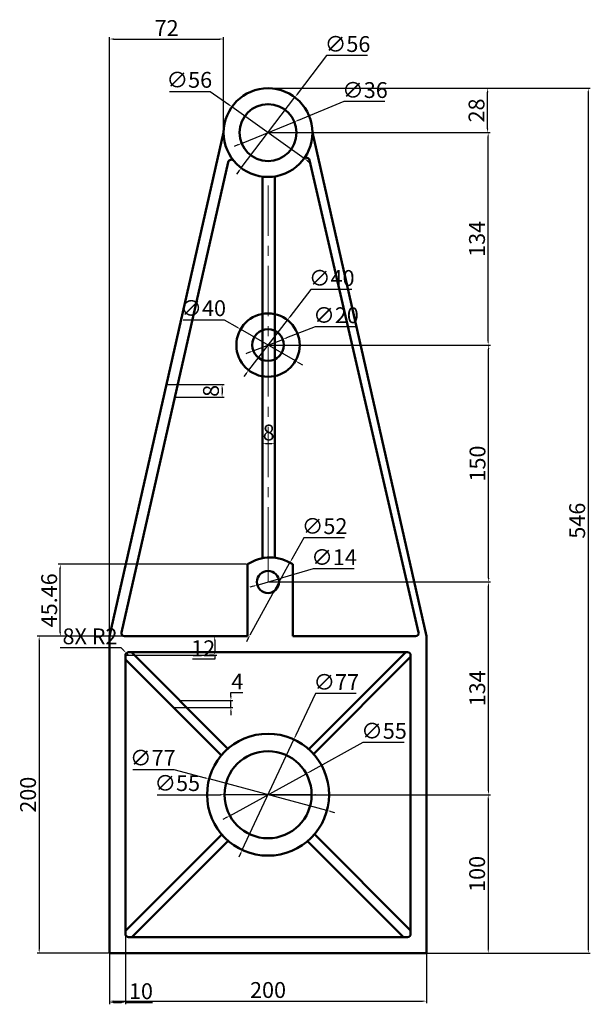
# Model space of a CAD drawing. Units: millimetres. Extents: x 2478 to 2838, y 972 to 1594.
import ezdxf

# ---------------------------------------------------------------- set-up
doc = ezdxf.new("R2010")
doc.units = ezdxf.units.MM
doc.linetypes.add('CENTER', pattern=[50.8, 31.75, -6.35, 6.35, -6.35])
for name, color, linetype, lineweight in [('M-CNTR', 4, 'CENTER', 18), ('M-DIMS', 2, 'Continuous', 25), ('M-OUTL', 7, 'Continuous', 50)]:
    doc.layers.add(name, color=color, linetype=linetype, lineweight=lineweight)
doc.styles.get("Standard").update_dxf_attribs({"font": 'arial.ttf'})
doc.dimstyles.new('ISO-25', dxfattribs={"dimtxt": 10, "dimasz": 2.5, "dimexe": 1.25, "dimexo": 0.625, "dimtad": 1, "dimtoh": 1, "dimdec": 0, "dimtxsty": 'Standard', "dimcen": 2.5, "dimadec": 0, "dimazin": 0, "dimtfac": 1, "dimtdec": 0, "dimtmove": 0, "dimatfit": 3, "dimfxl": 1, "dimarcsym": 0})

# ---------------------------------------------------------------- blocks, each defined once
blk = doc.blocks.new('*D1')
at = {"layer": 'Defpoints', "color": 0, "transparency": 16777216}
for p in [(2651.8, 1544.92), (2617.92, 1500.33)]:
    blk.add_point(p, dxfattribs=at)
at = {"layer": 'M-DIMS', "color": 0, "lineweight": -2, "transparency": 16777216}
for p, q in [((2671.81, 1571.25), (2653.31, 1546.91)), ((2697.63, 1571.25), (2671.81, 1571.25)), ((2617.92, 1500.33), (2651.8, 1544.92)), ((2616.4, 1498.34), (2614.89, 1496.35))]:
    blk.add_line(p, q, dxfattribs=at)
at = {"layer": 'M-DIMS', "color": 0, "transparency": 16777216}
for points in [[(2652.98, 1547.16), (2653.65, 1546.66), (2651.8, 1544.92)], [(2616.07, 1498.59), (2616.74, 1498.09), (2617.92, 1500.33)]]:
    blk.add_solid(points, dxfattribs=at)
at = {"layer": 'M-DIMS', "color": 0, "transparency": 16777216, "insert": (2685.04, 1577.26), "char_height": 10, "attachment_point": 5}
blk.add_mtext('∅56', dxfattribs=at)
blk = doc.blocks.new('*D2')
at = {"layer": 'Defpoints', "color": 0, "transparency": 16777216}
for p in [(2651.52, 1529.43), (2618.2, 1515.82)]:
    blk.add_point(p, dxfattribs=at)
at = {"layer": 'M-DIMS', "color": 0, "lineweight": -2, "transparency": 16777216}
for p, q in [((2682.79, 1542.2), (2653.84, 1530.38)), ((2708.61, 1542.2), (2682.79, 1542.2)), ((2618.2, 1515.82), (2651.52, 1529.43)), ((2615.88, 1514.87), (2613.57, 1513.93))]:
    blk.add_line(p, q, dxfattribs=at)
at = {"layer": 'M-DIMS', "color": 0, "transparency": 16777216}
for points in [[(2653.68, 1530.76), (2653.99, 1529.99), (2651.52, 1529.43)], [(2615.72, 1515.26), (2616.04, 1514.49), (2618.2, 1515.82)]]:
    blk.add_solid(points, dxfattribs=at)
at = {"layer": 'M-DIMS', "color": 0, "transparency": 16777216, "insert": (2696.01, 1548.21), "char_height": 10, "attachment_point": 5}
blk.add_mtext('∅36', dxfattribs=at)
blk = doc.blocks.new('*D3')
at = {"layer": 'Defpoints', "color": 0, "transparency": 16777216}
for p in [(2647.06, 1404.32), (2622.66, 1372.63)]:
    blk.add_point(p, dxfattribs=at)
at = {"layer": 'M-DIMS', "color": 0, "lineweight": -2, "transparency": 16777216}
for p, q in [((2661.86, 1423.53), (2648.59, 1406.3)), ((2687.65, 1423.53), (2661.86, 1423.53)), ((2622.66, 1372.63), (2647.06, 1404.32)), ((2621.13, 1370.65), (2619.61, 1368.67))]:
    blk.add_line(p, q, dxfattribs=at)
at = {"layer": 'M-DIMS', "color": 0, "transparency": 16777216}
for points in [[(2648.26, 1406.56), (2648.92, 1406.05), (2647.06, 1404.32)], [(2620.8, 1370.9), (2621.46, 1370.39), (2622.66, 1372.63)]]:
    blk.add_solid(points, dxfattribs=at)
at = {"layer": 'M-DIMS', "color": 0, "transparency": 16777216, "insert": (2675.07, 1429.54), "char_height": 10, "attachment_point": 5}
blk.add_mtext('∅40', dxfattribs=at)
blk = doc.blocks.new('*D4')
at = {"layer": 'Defpoints', "color": 0, "transparency": 16777216}
for p in [(2644.18, 1392.1), (2625.54, 1384.85)]:
    blk.add_point(p, dxfattribs=at)
at = {"layer": 'M-DIMS', "color": 0, "lineweight": -2, "transparency": 16777216}
for p, q in [((2664.54, 1400.03), (2646.51, 1393.01)), ((2690.33, 1400.03), (2664.54, 1400.03)), ((2625.54, 1384.85), (2644.18, 1392.1)), ((2623.21, 1383.94), (2620.88, 1383.03))]:
    blk.add_line(p, q, dxfattribs=at)
at = {"layer": 'M-DIMS', "color": 0, "transparency": 16777216}
for points in [[(2646.36, 1393.4), (2646.66, 1392.62), (2644.18, 1392.1)], [(2623.06, 1384.33), (2623.36, 1383.55), (2625.54, 1384.85)]]:
    blk.add_solid(points, dxfattribs=at)
at = {"layer": 'M-DIMS', "color": 0, "transparency": 16777216, "insert": (2677.75, 1406.04), "char_height": 10, "attachment_point": 5}
blk.add_mtext('∅20', dxfattribs=at)
blk = doc.blocks.new('*D5')
at = {"layer": 'Defpoints', "color": 0, "transparency": 16777216}
for p in [(2648.7, 1251.13), (2623.6, 1205.59)]:
    blk.add_point(p, dxfattribs=at)
at = {"layer": 'M-DIMS', "color": 0, "lineweight": -2, "transparency": 16777216}
for p, q in [((2657.37, 1266.87), (2649.9, 1253.32)), ((2683.1, 1266.87), (2657.37, 1266.87)), ((2623.6, 1205.59), (2648.7, 1251.13)), ((2622.39, 1203.4), (2621.18, 1201.21))]:
    blk.add_line(p, q, dxfattribs=at)
at = {"layer": 'M-DIMS', "color": 0, "transparency": 16777216}
for points in [[(2649.54, 1253.52), (2650.27, 1253.12), (2648.7, 1251.13)], [(2622.03, 1203.6), (2622.76, 1203.2), (2623.6, 1205.59)]]:
    blk.add_solid(points, dxfattribs=at)
at = {"layer": 'M-DIMS', "color": 0, "transparency": 16777216, "insert": (2670.55, 1272.88), "char_height": 10, "attachment_point": 5}
blk.add_mtext('∅52', dxfattribs=at)
blk = doc.blocks.new('*D6')
at = {"layer": 'Defpoints', "color": 0, "transparency": 16777216}
for p in [(2641.62, 1240.9), (2628.1, 1236.95)]:
    blk.add_point(p, dxfattribs=at)
at = {"layer": 'M-DIMS', "color": 0, "lineweight": -2, "transparency": 16777216}
for p, q in [((2663.33, 1247.23), (2644.02, 1241.6)), ((2689.12, 1247.23), (2663.33, 1247.23)), ((2628.1, 1236.95), (2641.62, 1240.9)), ((2625.7, 1236.25), (2623.3, 1235.55))]:
    blk.add_line(p, q, dxfattribs=at)
at = {"layer": 'M-DIMS', "color": 0, "transparency": 16777216}
for points in [[(2643.9, 1242), (2644.13, 1241.2), (2641.62, 1240.9)], [(2625.59, 1236.65), (2625.82, 1235.85), (2628.1, 1236.95)]]:
    blk.add_solid(points, dxfattribs=at)
at = {"layer": 'M-DIMS', "color": 0, "transparency": 16777216, "insert": (2676.53, 1253.24), "char_height": 10, "attachment_point": 5}
blk.add_mtext('∅14', dxfattribs=at)
blk = doc.blocks.new('*D7')
at = {"layer": 'Defpoints', "color": 0, "transparency": 16777216}
for p in [(2651.18, 1139.5), (2618.54, 1069.75)]:
    blk.add_point(p, dxfattribs=at)
at = {"layer": 'M-DIMS', "color": 0, "lineweight": -2, "transparency": 16777216}
for p, q in [((2664.71, 1168.41), (2652.24, 1141.76)), ((2690.53, 1168.41), (2664.71, 1168.41)), ((2618.54, 1069.75), (2651.18, 1139.5)), ((2617.48, 1067.49), (2616.42, 1065.22))]:
    blk.add_line(p, q, dxfattribs=at)
at = {"layer": 'M-DIMS', "color": 0, "transparency": 16777216}
for points in [[(2651.86, 1141.94), (2652.61, 1141.58), (2651.18, 1139.5)], [(2617.11, 1067.67), (2617.86, 1067.31), (2618.54, 1069.75)]]:
    blk.add_solid(points, dxfattribs=at)
at = {"layer": 'M-DIMS', "color": 0, "transparency": 16777216, "insert": (2677.93, 1174.42), "char_height": 10, "attachment_point": 5}
blk.add_mtext('∅77', dxfattribs=at)
blk = doc.blocks.new('*D8')
at = {"layer": 'Defpoints', "color": 0, "transparency": 16777216}
for p in [(2658.95, 1117.88), (2610.77, 1091.37)]:
    blk.add_point(p, dxfattribs=at)
at = {"layer": 'M-DIMS', "color": 0, "lineweight": -2, "transparency": 16777216}
for p, q in [((2694.78, 1137.6), (2661.14, 1119.09)), ((2720.68, 1137.6), (2694.78, 1137.6)), ((2610.77, 1091.37), (2658.95, 1117.88)), ((2608.58, 1090.16), (2606.39, 1088.96))]:
    blk.add_line(p, q, dxfattribs=at)
at = {"layer": 'M-DIMS', "color": 0, "transparency": 16777216}
for points in [[(2660.94, 1119.45), (2661.34, 1118.72), (2658.95, 1117.88)], [(2608.38, 1090.53), (2608.78, 1089.8), (2610.77, 1091.37)]]:
    blk.add_solid(points, dxfattribs=at)
at = {"layer": 'M-DIMS', "color": 0, "transparency": 16777216, "insert": (2708.04, 1143.61), "char_height": 10, "attachment_point": 5}
blk.add_mtext('∅55', dxfattribs=at)
blk = doc.blocks.new('*D9')
at = {"layer": 'Defpoints', "color": 0, "transparency": 16777216}
for p in [(2534.86, 1004.62), (2734.86, 1004.62), (2734.86, 974.28)]:
    blk.add_point(p, dxfattribs=at)
at = {"layer": 'M-DIMS', "color": 0, "lineweight": -2, "transparency": 16777216}
for p, q in [((2534.86, 1004), (2534.86, 973.03)), ((2734.86, 1004), (2734.86, 973.03)), ((2537.36, 974.28), (2732.36, 974.28))]:
    blk.add_line(p, q, dxfattribs=at)
at = {"layer": 'M-DIMS', "color": 0, "transparency": 16777216}
for points in [[(2537.36, 974.7), (2537.36, 973.86), (2534.86, 974.28)], [(2732.36, 974.7), (2732.36, 973.86), (2734.86, 974.28)]]:
    blk.add_solid(points, dxfattribs=at)
at = {"layer": 'M-DIMS', "color": 0, "transparency": 16777216, "insert": (2634.86, 980.01), "char_height": 10, "attachment_point": 5}
blk.add_mtext('200', dxfattribs=at)
blk = doc.blocks.new('*D10')
at = {"layer": 'Defpoints', "color": 0, "transparency": 16777216}
for p in [(2534.86, 1204.62), (2490.45, 1004.62), (2534.86, 1004.62)]:
    blk.add_point(p, dxfattribs=at)
at = {"layer": 'M-DIMS', "color": 0, "lineweight": -2, "transparency": 16777216}
for p, q in [((2534.23, 1204.62), (2489.2, 1204.62)), ((2490.45, 1202.12), (2490.45, 1007.12)), ((2534.23, 1004.62), (2489.2, 1004.62))]:
    blk.add_line(p, q, dxfattribs=at)
at = {"layer": 'M-DIMS', "color": 0, "transparency": 16777216}
for points in [[(2490.04, 1202.12), (2490.87, 1202.12), (2490.45, 1204.62)], [(2490.04, 1007.12), (2490.87, 1007.12), (2490.45, 1004.62)]]:
    blk.add_solid(points, dxfattribs=at)
at = {"layer": 'M-DIMS', "color": 0, "transparency": 16777216, "insert": (2484.72, 1104.62), "char_height": 10, "attachment_point": 5, "rotation": 90}
blk.add_mtext('200', dxfattribs=at)
blk = doc.blocks.new('*D11')
at = {"layer": 'Defpoints', "color": 0, "transparency": 16777216}
for p in [(2634.86, 1104.62), (2634.86, 1004.62), (2773.82, 1004.62)]:
    blk.add_point(p, dxfattribs=at)
at = {"layer": 'M-DIMS', "color": 0, "lineweight": -2, "transparency": 16777216}
for p, q in [((2635.48, 1104.62), (2775.07, 1104.62)), ((2773.82, 1102.12), (2773.82, 1007.12)), ((2635.48, 1004.62), (2775.07, 1004.62))]:
    blk.add_line(p, q, dxfattribs=at)
at = {"layer": 'M-DIMS', "color": 0, "transparency": 16777216}
for points in [[(2773.4, 1102.12), (2774.23, 1102.12), (2773.82, 1104.62)], [(2773.4, 1007.12), (2774.23, 1007.12), (2773.82, 1004.62)]]:
    blk.add_solid(points, dxfattribs=at)
at = {"layer": 'M-DIMS', "color": 0, "transparency": 16777216, "insert": (2768.09, 1054.62), "char_height": 10, "attachment_point": 5, "rotation": 90}
blk.add_mtext('100', dxfattribs=at)
blk = doc.blocks.new('*D12')
at = {"layer": 'Defpoints', "color": 0, "transparency": 16777216}
for p in [(2634.86, 1238.92), (2773.94, 1238.92), (2634.86, 1104.62)]:
    blk.add_point(p, dxfattribs=at)
at = {"layer": 'M-DIMS', "color": 0, "lineweight": -2, "transparency": 16777216}
for p, q in [((2635.48, 1238.92), (2775.19, 1238.92)), ((2773.94, 1107.12), (2773.94, 1236.42)), ((2635.48, 1104.62), (2775.19, 1104.62))]:
    blk.add_line(p, q, dxfattribs=at)
at = {"layer": 'M-DIMS', "color": 0, "transparency": 16777216}
for points in [[(2773.52, 1236.42), (2774.35, 1236.42), (2773.94, 1238.92)], [(2773.52, 1107.12), (2774.35, 1107.12), (2773.94, 1104.62)]]:
    blk.add_solid(points, dxfattribs=at)
at = {"layer": 'M-DIMS', "color": 0, "transparency": 16777216, "insert": (2768.2, 1171.77), "char_height": 10, "attachment_point": 5, "rotation": 90}
blk.add_mtext('134', dxfattribs=at)
blk = doc.blocks.new('*D13')
at = {"layer": 'Defpoints', "color": 0, "transparency": 16777216}
for p in [(2634.86, 1388.48), (2774.08, 1388.48), (2634.86, 1238.92)]:
    blk.add_point(p, dxfattribs=at)
at = {"layer": 'M-DIMS', "color": 0, "lineweight": -2, "transparency": 16777216}
for p, q in [((2635.48, 1388.48), (2775.33, 1388.48)), ((2774.08, 1241.42), (2774.08, 1385.98)), ((2635.48, 1238.92), (2775.33, 1238.92))]:
    blk.add_line(p, q, dxfattribs=at)
at = {"layer": 'M-DIMS', "color": 0, "transparency": 16777216}
for points in [[(2773.66, 1385.98), (2774.5, 1385.98), (2774.08, 1388.48)], [(2773.66, 1241.42), (2774.5, 1241.42), (2774.08, 1238.92)]]:
    blk.add_solid(points, dxfattribs=at)
at = {"layer": 'M-DIMS', "color": 0, "transparency": 16777216, "insert": (2768.35, 1313.7), "char_height": 10, "attachment_point": 5, "rotation": 90}
blk.add_mtext('150', dxfattribs=at)
blk = doc.blocks.new('*D14')
at = {"layer": 'Defpoints', "color": 0, "transparency": 16777216}
for p in [(2634.86, 1522.62), (2773.76, 1522.62), (2634.86, 1388.48)]:
    blk.add_point(p, dxfattribs=at)
at = {"layer": 'M-DIMS', "color": 0, "lineweight": -2, "transparency": 16777216}
for p, q in [((2635.48, 1522.62), (2775.01, 1522.62)), ((2773.76, 1390.98), (2773.76, 1520.12)), ((2635.48, 1388.48), (2775.01, 1388.48))]:
    blk.add_line(p, q, dxfattribs=at)
at = {"layer": 'M-DIMS', "color": 0, "transparency": 16777216}
for points in [[(2773.34, 1520.12), (2774.17, 1520.12), (2773.76, 1522.62)], [(2773.34, 1390.98), (2774.17, 1390.98), (2773.76, 1388.48)]]:
    blk.add_solid(points, dxfattribs=at)
at = {"layer": 'M-DIMS', "color": 0, "transparency": 16777216, "insert": (2768.02, 1455.55), "char_height": 10, "attachment_point": 5, "rotation": 90}
blk.add_mtext('134', dxfattribs=at)
blk = doc.blocks.new('*D15')
at = {"layer": 'Defpoints', "color": 0, "transparency": 16777216}
for p in [(2634.86, 1550.62), (2773.43, 1550.62), (2634.86, 1522.62)]:
    blk.add_point(p, dxfattribs=at)
at = {"layer": 'M-DIMS', "color": 0, "lineweight": -2, "transparency": 16777216}
for p, q in [((2635.48, 1550.62), (2774.68, 1550.62)), ((2773.43, 1525.12), (2773.43, 1548.12)), ((2635.48, 1522.62), (2774.68, 1522.62))]:
    blk.add_line(p, q, dxfattribs=at)
at = {"layer": 'M-DIMS', "color": 0, "transparency": 16777216}
for points in [[(2773.01, 1548.12), (2773.85, 1548.12), (2773.43, 1550.62)], [(2773.01, 1525.12), (2773.85, 1525.12), (2773.43, 1522.62)]]:
    blk.add_solid(points, dxfattribs=at)
at = {"layer": 'M-DIMS', "color": 0, "transparency": 16777216, "insert": (2767.7, 1536.62), "char_height": 10, "attachment_point": 5, "rotation": 90}
blk.add_mtext('28', dxfattribs=at)
blk = doc.blocks.new('*D16')
at = {"layer": 'Defpoints', "color": 0, "transparency": 16777216}
for p in [(2634.86, 1550.62), (2634.86, 1004.62), (2836.96, 1004.62)]:
    blk.add_point(p, dxfattribs=at)
at = {"layer": 'M-DIMS', "color": 0, "lineweight": -2, "transparency": 16777216}
for p, q in [((2635.48, 1550.62), (2838.21, 1550.62)), ((2836.96, 1548.12), (2836.96, 1007.12)), ((2635.48, 1004.62), (2838.21, 1004.62))]:
    blk.add_line(p, q, dxfattribs=at)
at = {"layer": 'M-DIMS', "color": 0, "transparency": 16777216}
for points in [[(2836.54, 1548.12), (2837.38, 1548.12), (2836.96, 1550.62)], [(2836.54, 1007.12), (2837.38, 1007.12), (2836.96, 1004.62)]]:
    blk.add_solid(points, dxfattribs=at)
at = {"layer": 'M-DIMS', "color": 0, "transparency": 16777216, "insert": (2831.23, 1277.62), "char_height": 10, "attachment_point": 5, "rotation": 90}
blk.add_mtext('546', dxfattribs=at)
blk = doc.blocks.new('*D17')
at = {"layer": 'Defpoints', "color": 0, "transparency": 16777216}
for p in [(2570.86, 1363.62), (2576.07, 1355.55), (2605.87, 1355.55)]:
    blk.add_point(p, dxfattribs=at)
at = {"layer": 'M-DIMS', "color": 0, "lineweight": -2, "transparency": 16777216}
for p, q in [((2571.48, 1363.62), (2607.12, 1363.62)), ((2576.69, 1355.55), (2607.12, 1355.55)), ((2605.87, 1361.12), (2605.87, 1358.05))]:
    blk.add_line(p, q, dxfattribs=at)
at = {"layer": 'M-DIMS', "color": 0, "transparency": 16777216}
for points in [[(2605.45, 1361.12), (2606.29, 1361.12), (2605.87, 1363.62)], [(2605.45, 1358.05), (2606.29, 1358.05), (2605.87, 1355.55)]]:
    blk.add_solid(points, dxfattribs=at)
at = {"layer": 'M-DIMS', "color": 0, "transparency": 16777216, "insert": (2600.14, 1359.59), "char_height": 10, "attachment_point": 5, "rotation": 90}
blk.add_mtext('8', dxfattribs=at)
blk = doc.blocks.new('*D18')
at = {"layer": 'Defpoints', "color": 0, "transparency": 16777216}
for p in [(2631.31, 1374.59), (2639.25, 1374.65), (2639.25, 1326.25)]:
    blk.add_point(p, dxfattribs=at)
at = {"layer": 'M-DIMS', "color": 0, "lineweight": -2, "transparency": 16777216}
for p, q in [((2631.31, 1373.96), (2631.31, 1325)), ((2639.25, 1374.02), (2639.25, 1325)), ((2633.81, 1326.25), (2636.75, 1326.25))]:
    blk.add_line(p, q, dxfattribs=at)
at = {"layer": 'M-DIMS', "color": 0, "transparency": 16777216}
for points in [[(2633.81, 1326.66), (2633.81, 1325.83), (2631.31, 1326.25)], [(2636.75, 1326.66), (2636.75, 1325.83), (2639.25, 1326.25)]]:
    blk.add_solid(points, dxfattribs=at)
at = {"layer": 'M-DIMS', "color": 0, "transparency": 16777216, "insert": (2635.28, 1331.98), "char_height": 10, "attachment_point": 5}
blk.add_mtext('8', dxfattribs=at)
blk = doc.blocks.new('*D19')
at = {"layer": 'Defpoints', "color": 0, "transparency": 16777216}
for p in [(2579.1, 1164.14), (2611.44, 1164.14), (2575.15, 1159.75)]:
    blk.add_point(p, dxfattribs=at)
at = {"layer": 'M-DIMS', "color": 0, "lineweight": -2, "transparency": 16777216}
for p, q in [((2611.44, 1166.64), (2611.44, 1169.14)), ((2611.44, 1169.14), (2618.98, 1169.14)), ((2579.72, 1164.14), (2612.69, 1164.14)), ((2611.44, 1159.75), (2611.44, 1164.14)), ((2575.77, 1159.75), (2612.69, 1159.75)), ((2611.44, 1157.25), (2611.44, 1154.75))]:
    blk.add_line(p, q, dxfattribs=at)
at = {"layer": 'M-DIMS', "color": 0, "transparency": 16777216}
for points in [[(2611.02, 1166.64), (2611.85, 1166.64), (2611.44, 1164.14)], [(2611.02, 1157.25), (2611.85, 1157.25), (2611.44, 1159.75)]]:
    blk.add_solid(points, dxfattribs=at)
at = {"layer": 'M-DIMS', "color": 0, "transparency": 16777216, "insert": (2615.52, 1174.77), "char_height": 10, "attachment_point": 5}
blk.add_mtext('4', dxfattribs=at)
blk = doc.blocks.new('*D20')
at = {"layer": 'Defpoints', "color": 0, "transparency": 16777216}
for p in [(2542.8, 1204.62), (2544.86, 1192.62), (2601.2, 1192.62)]:
    blk.add_point(p, dxfattribs=at)
at = {"layer": 'M-DIMS', "color": 0, "lineweight": -2, "transparency": 16777216}
for p, q in [((2543.43, 1204.62), (2602.45, 1204.62)), ((2601.2, 1202.12), (2601.2, 1195.12)), ((2545.48, 1192.62), (2602.45, 1192.62)), ((2601.2, 1190.12), (2587.3, 1190.12)), ((2601.2, 1192.62), (2601.2, 1190.12))]:
    blk.add_line(p, q, dxfattribs=at)
at = {"layer": 'M-DIMS', "color": 0, "transparency": 16777216}
for points in [[(2600.79, 1202.12), (2601.62, 1202.12), (2601.2, 1204.62)], [(2600.79, 1195.12), (2601.62, 1195.12), (2601.2, 1192.62)]]:
    blk.add_solid(points, dxfattribs=at)
at = {"layer": 'M-DIMS', "color": 0, "transparency": 16777216, "insert": (2593.94, 1195.77), "char_height": 10, "attachment_point": 5}
blk.add_mtext('12', dxfattribs=at)
blk = doc.blocks.new('*D21')
at = {"layer": 'Defpoints', "color": 0, "transparency": 16777216}
for p in [(2606.86, 1581.72), (2606.86, 1522.62), (2534.86, 1204.62)]:
    blk.add_point(p, dxfattribs=at)
at = {"layer": 'M-DIMS', "color": 0, "lineweight": -2, "transparency": 16777216}
for p, q in [((2534.86, 1205.25), (2534.86, 1582.97)), ((2537.36, 1581.72), (2604.36, 1581.72)), ((2606.86, 1523.25), (2606.86, 1582.97))]:
    blk.add_line(p, q, dxfattribs=at)
at = {"layer": 'M-DIMS', "color": 0, "transparency": 16777216}
for points in [[(2537.36, 1582.14), (2537.36, 1581.31), (2534.86, 1581.72)], [(2604.36, 1582.14), (2604.36, 1581.31), (2606.86, 1581.72)]]:
    blk.add_solid(points, dxfattribs=at)
at = {"layer": 'M-DIMS', "color": 0, "transparency": 16777216, "insert": (2570.86, 1587.37), "char_height": 10, "attachment_point": 5}
blk.add_mtext('72', dxfattribs=at)
blk = doc.blocks.new('*D22')
at = {"layer": 'Defpoints', "color": 0, "transparency": 16777216}
for p in [(2503.76, 1250.08), (2621.86, 1250.08), (2621.86, 1204.62)]:
    blk.add_point(p, dxfattribs=at)
at = {"layer": 'M-DIMS', "color": 0, "lineweight": -2, "transparency": 16777216}
for p, q in [((2621.23, 1250.08), (2502.51, 1250.08)), ((2503.76, 1207.12), (2503.76, 1247.58)), ((2621.23, 1204.62), (2502.51, 1204.62))]:
    blk.add_line(p, q, dxfattribs=at)
at = {"layer": 'M-DIMS', "color": 0, "transparency": 16777216}
for points in [[(2503.34, 1247.58), (2504.18, 1247.58), (2503.76, 1250.08)], [(2503.34, 1207.12), (2504.18, 1207.12), (2503.76, 1204.62)]]:
    blk.add_solid(points, dxfattribs=at)
at = {"layer": 'M-DIMS', "color": 0, "transparency": 16777216, "insert": (2498.03, 1227.35), "char_height": 10, "attachment_point": 5, "rotation": 90}
blk.add_mtext('45.46', dxfattribs=at)
blk = doc.blocks.new('*D23')
at = {"layer": 'Defpoints', "color": 0, "transparency": 16777216}
for p in [(2534.86, 1204.62), (2544.86, 1192.62), (2544.86, 973.52)]:
    blk.add_point(p, dxfattribs=at)
at = {"layer": 'M-DIMS', "color": 0, "lineweight": -2, "transparency": 16777216}
for p, q in [((2534.86, 1204), (2534.86, 972.27)), ((2544.86, 1192), (2544.86, 972.27)), ((2537.36, 973.52), (2542.36, 973.52)), ((2544.86, 973.52), (2561.96, 973.52))]:
    blk.add_line(p, q, dxfattribs=at)
at = {"layer": 'M-DIMS', "color": 0, "transparency": 16777216}
for points in [[(2537.36, 973.94), (2537.36, 973.11), (2534.86, 973.52)], [(2542.36, 973.94), (2542.36, 973.11), (2544.86, 973.52)]]:
    blk.add_solid(points, dxfattribs=at)
at = {"layer": 'M-DIMS', "color": 0, "transparency": 16777216, "insert": (2554.66, 979.26), "char_height": 10, "attachment_point": 5}
blk.add_mtext('10', dxfattribs=at)
blk = doc.blocks.new('*D24')
at = {"layer": 'Defpoints', "color": 0, "transparency": 16777216}
for p in [(2607.36, 1104.62), (2662.36, 1104.62)]:
    blk.add_point(p, dxfattribs=at)
at = {"layer": 'M-DIMS', "color": 0, "lineweight": -2, "transparency": 16777216}
for p, q in [((2564.95, 1104.63), (2590.86, 1104.63)), ((2590.86, 1104.63), (2604.86, 1104.62)), ((2662.36, 1104.62), (2607.36, 1104.62)), ((2664.86, 1104.62), (2667.36, 1104.62))]:
    blk.add_line(p, q, dxfattribs=at)
at = {"layer": 'M-DIMS', "color": 0, "transparency": 16777216}
for points in [[(2604.86, 1105.04), (2604.86, 1104.21), (2607.36, 1104.62)], [(2664.86, 1105.04), (2664.86, 1104.21), (2662.36, 1104.62)]]:
    blk.add_solid(points, dxfattribs=at)
at = {"layer": 'M-DIMS', "color": 0, "transparency": 16777216, "insert": (2577.59, 1110.64), "char_height": 10, "attachment_point": 5}
blk.add_mtext('∅55', dxfattribs=at)
blk = doc.blocks.new('*D25')
at = {"layer": 'Defpoints', "color": 0, "transparency": 16777216}
for p in [(2597.67, 1114.59), (2672.05, 1094.66)]:
    blk.add_point(p, dxfattribs=at)
at = {"layer": 'M-DIMS', "color": 0, "lineweight": -2, "transparency": 16777216}
for p, q in [((2549.53, 1120.57), (2575.36, 1120.57)), ((2575.36, 1120.57), (2595.26, 1115.24)), ((2672.05, 1094.66), (2597.67, 1114.59)), ((2674.46, 1094.01), (2676.88, 1093.37))]:
    blk.add_line(p, q, dxfattribs=at)
at = {"layer": 'M-DIMS', "color": 0, "transparency": 16777216}
for points in [[(2595.36, 1115.64), (2595.15, 1114.83), (2597.67, 1114.59)], [(2674.57, 1094.41), (2674.35, 1093.61), (2672.05, 1094.66)]]:
    blk.add_solid(points, dxfattribs=at)
at = {"layer": 'M-DIMS', "color": 0, "transparency": 16777216, "insert": (2562.13, 1126.58), "char_height": 10, "attachment_point": 5}
blk.add_mtext('∅77', dxfattribs=at)
blk = doc.blocks.new('*D26')
at = {"layer": 'Defpoints', "color": 0, "transparency": 16777216}
for p in [(2617.54, 1398.48), (2652.18, 1378.47)]:
    blk.add_point(p, dxfattribs=at)
at = {"layer": 'M-DIMS', "color": 0, "lineweight": -2, "transparency": 16777216}
for p, q in [((2581.35, 1404.48), (2607.15, 1404.48)), ((2607.15, 1404.48), (2615.37, 1399.73)), ((2652.18, 1378.47), (2617.54, 1398.48)), ((2654.34, 1377.22), (2656.51, 1375.97))]:
    blk.add_line(p, q, dxfattribs=at)
at = {"layer": 'M-DIMS', "color": 0, "transparency": 16777216}
for points in [[(2615.58, 1400.09), (2615.17, 1399.37), (2617.54, 1398.48)], [(2654.55, 1377.59), (2654.14, 1376.86), (2652.18, 1378.47)]]:
    blk.add_solid(points, dxfattribs=at)
at = {"layer": 'M-DIMS', "color": 0, "transparency": 16777216, "insert": (2593.94, 1410.49), "char_height": 10, "attachment_point": 5}
blk.add_mtext('∅40', dxfattribs=at)
blk = doc.blocks.new('*D27')
at = {"layer": 'Defpoints', "color": 0, "transparency": 16777216}
for p in [(2612.07, 1538.9), (2657.65, 1506.35)]:
    blk.add_point(p, dxfattribs=at)
at = {"layer": 'M-DIMS', "color": 0, "lineweight": -2, "transparency": 16777216}
for p, q in [((2572.58, 1548.66), (2598.4, 1548.66)), ((2598.4, 1548.66), (2610.04, 1540.35)), ((2657.65, 1506.35), (2612.07, 1538.9)), ((2659.68, 1504.9), (2661.72, 1503.45))]:
    blk.add_line(p, q, dxfattribs=at)
at = {"layer": 'M-DIMS', "color": 0, "transparency": 16777216}
for points in [[(2610.28, 1540.69), (2609.8, 1540.01), (2612.07, 1538.9)], [(2659.92, 1505.24), (2659.44, 1504.56), (2657.65, 1506.35)]]:
    blk.add_solid(points, dxfattribs=at)
at = {"layer": 'M-DIMS', "color": 0, "transparency": 16777216, "insert": (2585.18, 1554.67), "char_height": 10, "attachment_point": 5}
blk.add_mtext('∅56', dxfattribs=at)
blk = doc.blocks.new('*D28')
at = {"layer": 'Defpoints', "color": 0, "transparency": 16777216}
for p in [(2545.45, 1194.04), (2546.86, 1192.62)]:
    blk.add_point(p, dxfattribs=at)
at = {"layer": 'M-DIMS', "color": 0, "lineweight": -2, "transparency": 16777216}
for p, q in [((2503.76, 1197.58), (2541.91, 1197.58)), ((2541.91, 1197.58), (2543.68, 1195.81)), ((2546.86, 1192.62), (2545.45, 1194.04))]:
    blk.add_line(p, q, dxfattribs=at)
at = {"layer": 'M-DIMS', "color": 0, "transparency": 16777216}
blk.add_solid([(2543.97, 1196.1), (2543.38, 1195.51), (2545.45, 1194.04)], dxfattribs=at)
at = {"layer": 'M-DIMS', "color": 0, "transparency": 16777216, "insert": (2522.52, 1203.31), "char_height": 10, "attachment_point": 5}
blk.add_mtext('8X R2', dxfattribs=at)

msp = doc.modelspace()

# ---------------------------------------------------------------- linework, layer by layer
at = {"layer": 'M-CNTR'}
for q in [(2634.86, 1494.625), (2634.86, 1238.923)]:
    msp.add_line((2634.86, 1254.327), q, dxfattribs=at)
at = {"layer": 'M-OUTL'}
for p, q in [((2534.86, 1204.625), (2606.86, 1522.625)), ((2734.86, 1204.625), (2662.86, 1522.625)), ((2729.869, 1207.075), (2660.962, 1505.282)), ((2542.413, 1207.067), (2609.72, 1504.033)), ((2631.307, 1254.327), (2631.307, 1494.851)), ((2639.25, 1254.327), (2639.25, 1494.971)), ((2621.86, 1204.625), (2621.86, 1250.081)), ((2650.436, 1250.081), (2650.436, 1204.625)), ((2534.86, 1004.625), (2534.86, 1204.625)), ((2621.86, 1204.625), (2544.364, 1204.625)), ((2650.436, 1204.625), (2727.921, 1204.625)), ((2734.86, 1204.625), (2734.86, 1004.625)), ((2548.617, 1194.625), (2546.86, 1194.625)), ((2721.86, 1194.625), (2548.617, 1194.625)), ((2548.617, 1194.625), (2609.58, 1133.662)), ((2660.542, 1133.307), (2721.86, 1194.625)), ((2721.86, 1194.625), (2722.86, 1194.625)), ((2544.86, 1190.035), (2544.86, 1192.625)), ((2544.86, 1190.035), (2605.438, 1129.456)), ((2544.86, 1190.035), (2544.86, 1018.751)), ((2663.542, 1130.307), (2724.86, 1191.625)), ((2724.86, 1191.625), (2724.86, 1192.625)), ((2724.86, 1018.937), (2724.86, 1191.625)), ((2544.86, 1018.751), (2605.651, 1079.542)), ((2664.154, 1079.643), (2724.86, 1018.937)), ((2548.985, 1014.625), (2609.777, 1075.417)), ((2659.695, 1075.206), (2720.277, 1014.625)), ((2544.86, 1018.751), (2544.86, 1016.625)), ((2548.985, 1014.625), (2546.86, 1014.625)), ((2548.985, 1014.625), (2720.277, 1014.625)), ((2720.277, 1014.625), (2722.86, 1014.625)), ((2724.86, 1018.937), (2724.86, 1016.625)), ((2734.86, 1004.625), (2534.86, 1004.625))]:
    msp.add_line(p, q, dxfattribs=at)
for centre, radius in [((2634.86, 1522.625), 28), ((2634.86, 1522.625), 18), ((2634.86, 1388.476), 20), ((2634.86, 1388.476), 10), ((2634.86, 1238.923), 7.038), ((2634.86, 1104.625), 38.5), ((2634.86, 1104.625), 27.5)]:
    msp.add_circle(centre, radius, dxfattribs=at)
for centre, radius, start, end in [((2611.67, 1503.591), 2, 39.37847, 167.229795), ((2659.013, 1504.832), 2, 13.01111, 143.622803), ((2636.148, 1228.359), 26, 56.664415, 123.335585), ((2544.364, 1206.625), 2, 167.229795, 270), ((2727.921, 1206.625), 2, 270, 13.01111), ((2546.86, 1192.625), 2, 90, 180), ((2722.86, 1192.625), 2, 0, 90), ((2546.86, 1016.625), 2, 180, 270), ((2722.86, 1016.625), 2, 270, 0)]:
    msp.add_arc(centre, radius, start, end, dxfattribs=at)

# ---------------------------------------------------------------- dimensions: what is measured, and where the dimension line sits
at = {"layer": 'M-DIMS'}
for base, p1, p2, override, picture, middle in [((2606.86, 1581.725), (2534.86, 1204.625), (2606.86, 1522.625), {"dimdec": 0, "dimlfac": 1, "dimrnd": 0, "dimzin": 0, "dimdsep": 46, "dimlunit": 2}, '*D21', (2570.86, 1587.37)), ((2639.25, 1326.246), (2631.307, 1374.589), (2639.25, 1374.649), {"dimclrd": 0, "dimclre": 0, "dimclrt": 0}, '*D18', (2635.278, 1331.977)), ((2544.86, 973.525), (2534.86, 1204.625), (2544.86, 1192.625), {"dimdec": 0, "dimlfac": 1, "dimrnd": 0, "dimzin": 0, "dimdsep": 46, "dimlunit": 2}, '*D23', (2554.659, 979.255)), ((2734.86, 974.281), (2534.86, 1004.625), (2734.86, 1004.625), {"dimclrd": 0, "dimclre": 0, "dimclrt": 0}, '*D9', (2634.86, 980.012))]:
    dim = msp.add_linear_dim(base=base, p1=p1, p2=p2, dimstyle='ISO-25', override=override, dxfattribs=at)
    dim.commit()
    dim.dimension.update_dxf_attribs({"geometry": picture, "text_midpoint": middle})
for p1, p2, override, picture, middle in [((2617.917, 1500.332), (2651.802, 1544.917), {"dimclrd": 0, "dimclre": 0, "dimclrt": 0}, '*D1', (2685.036, 1571.245)), ((2657.647, 1506.354), (2612.072, 1538.895), {"dimdec": 0, "dimlfac": 1, "dimrnd": 0, "dimzin": 0, "dimdsep": 46, "dimlunit": 2}, '*D27', (2585.176, 1548.658)), ((2618.196, 1515.818), (2651.523, 1529.431), {"dimclrd": 0, "dimclre": 0, "dimclrt": 0}, '*D2', (2696.011, 1542.202)), ((2622.657, 1372.63), (2647.062, 1404.322), {"dimclrd": 0, "dimclre": 0, "dimclrt": 0}, '*D3', (2675.067, 1423.534)), ((2652.18, 1378.475), (2617.539, 1398.476), {"dimdec": 0, "dimlfac": 1, "dimrnd": 0, "dimzin": 0, "dimdsep": 46, "dimlunit": 2}, '*D26', (2593.937, 1404.477)), ((2625.541, 1384.847), (2644.178, 1392.104), {"dimclrd": 0, "dimclre": 0, "dimclrt": 0}, '*D4', (2677.747, 1400.031)), ((2623.598, 1205.588), (2648.698, 1251.129), {"dimclrd": 0, "dimclre": 0, "dimclrt": 0}, '*D5', (2670.549, 1266.868)), ((2628.104, 1236.952), (2641.615, 1240.895), {"dimclrd": 0, "dimclre": 0, "dimclrt": 0}, '*D6', (2676.535, 1247.233)), ((2618.543, 1069.753), (2651.176, 1139.496), {"dimclrd": 0, "dimclre": 0, "dimclrt": 0}, '*D7', (2677.933, 1168.41)), ((2610.767, 1091.366), (2658.952, 1117.883), {"dimclrd": 0, "dimclre": 0, "dimclrt": 0}, '*D8', (2708.04, 1137.596)), ((2672.048, 1094.66), (2597.672, 1114.59), {"dimdec": 0, "dimlfac": 1, "dimrnd": 0, "dimzin": 0, "dimdsep": 46, "dimlunit": 2}, '*D25', (2562.131, 1120.569)), ((2662.36, 1104.624), (2607.36, 1104.625), {"dimdec": 0, "dimlfac": 1, "dimrnd": 0, "dimzin": 0, "dimdsep": 46, "dimlunit": 2}, '*D24', (2590.86, 1104.625))]:
    dim = msp.add_diameter_dim_2p(p1=p1, p2=p2, dimstyle='ISO-25', override=override, dxfattribs=at)
    dim.commit()
    dim.dimension.update_dxf_attribs({"geometry": picture, "text_midpoint": middle, "dimtype": 163})
for base, p1, p2, override, picture, middle in [((2773.429, 1550.625), (2634.86, 1522.625), (2634.86, 1550.625), {"dimclrd": 0, "dimclre": 0, "dimclrt": 0}, '*D15', (2767.699, 1536.625)), ((2836.96, 1004.625), (2634.86, 1550.625), (2634.86, 1004.625), {"dimclrd": 0, "dimclre": 0, "dimclrt": 0}, '*D16', (2831.23, 1277.625)), ((2773.756, 1522.625), (2634.86, 1388.476), (2634.86, 1522.625), {"dimclrd": 0, "dimclre": 0, "dimclrt": 0}, '*D14', (2768.021, 1455.55)), ((2774.078, 1388.476), (2634.86, 1238.923), (2634.86, 1388.476), {"dimclrd": 0, "dimclre": 0, "dimclrt": 0}, '*D13', (2768.348, 1313.7)), ((2605.87, 1355.55), (2570.86, 1363.625), (2576.066, 1355.55), {"dimclrd": 0, "dimclre": 0, "dimclrt": 0}, '*D17', (2600.14, 1359.587)), ((2503.76, 1250.081), (2621.86, 1204.625), (2621.86, 1250.081), {"dimdec": 2, "dimlfac": 1, "dimrnd": 0, "dimzin": 0, "dimdsep": 46, "dimlunit": 2}, '*D22', (2498.029, 1227.353)), ((2773.937, 1238.923), (2634.86, 1104.625), (2634.86, 1238.923), {"dimclrd": 0, "dimclre": 0, "dimclrt": 0}, '*D12', (2768.203, 1171.774)), ((2490.453, 1004.625), (2534.86, 1204.625), (2534.86, 1004.625), {"dimclrd": 0, "dimclre": 0, "dimclrt": 0}, '*D10', (2484.723, 1104.625)), ((2601.202, 1192.625), (2542.801, 1204.625), (2544.86, 1192.625), {"dimclrd": 0, "dimclre": 0, "dimclrt": 0}, '*D20', (2593.936, 1195.77)), ((2611.438, 1164.143), (2575.149, 1159.746), (2579.099, 1164.143), {"dimclrd": 0, "dimclre": 0, "dimclrt": 0}, '*D19', (2615.522, 1174.768)), ((2773.817, 1004.625), (2634.86, 1104.625), (2634.86, 1004.625), {"dimclrd": 0, "dimclre": 0, "dimclrt": 0}, '*D11', (2768.087, 1054.625))]:
    dim = msp.add_linear_dim(base=base, p1=p1, p2=p2, angle=90, dimstyle='ISO-25', override=override, dxfattribs=at)
    dim.commit()
    dim.dimension.update_dxf_attribs({"geometry": picture, "text_midpoint": middle})
dim = msp.add_radius_dim(center=(2546.86, 1192.625), mpoint=(2545.446, 1194.039), text='8X <>', dimstyle='ISO-25', override={"dimdec": 0, "dimlfac": 1, "dimrnd": 0, "dimzin": 0, "dimdsep": 46, "dimlunit": 2}, dxfattribs=at)
dim.commit()
dim.dimension.update_dxf_attribs({"geometry": '*D28', "text_midpoint": (2522.524, 1203.307)})

doc.saveas('drawing.dxf')
